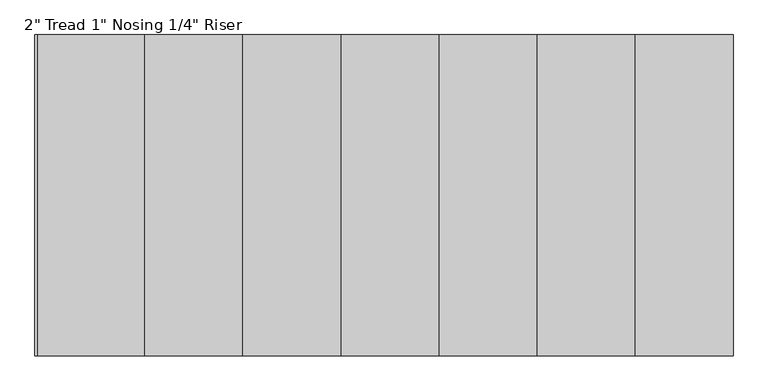
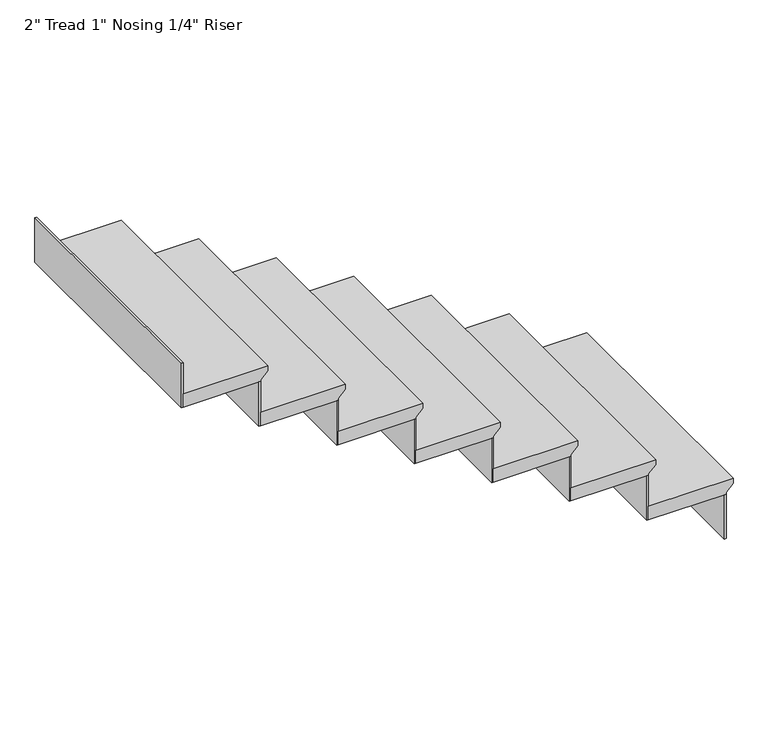
"""IFC4 building model written with IfcOpenShell, lengths in millimetres: stair flight geometry."""

from ifc_helpers import new_model, si_unit, frame, origin, place, context, project, spatial, polyline, outline, extrude, source, transform, mapped, element, save


def stair_flight_81020766(model_context):
    return source(origin(), model_context, "Body", "SweptSolid", [
        extrude(outline(polyline([(1862.6666667, -3900.6725091), (1862.6666667, -4205.4725091), (1811.8666667, -4205.4725091), (1811.8666667, -3926.0725091), (1818.2166667, -3926.0725091), (1843.6166667, -3900.6725091), (1862.6666667, -3900.6725091)])), frame((0.0, 8912.1149226, 0.0), z_axis=(0.0, 1.0, 0.0), x_axis=(0.0, 0.0, 1.0)), (0.0, 0.0, 1.0), 914.4),
        extrude(outline(polyline([(-3932.4225091, 9826.5149226), (-3926.0725091, 9826.5149226), (-3926.0725091, 8912.1149226), (-3932.4225091, 8912.1149226), (-3932.4225091, 9826.5149226)])), frame((0.0, 0.0, 1642.5333333), z_axis=(0.0, 0.0, 1.0), x_axis=(1.0, 0.0, 0.0)), (0.0, 0.0, 1.0), 169.3333333),
        extrude(outline(polyline([(-4211.8225091, 9826.5149226), (-4205.4725091, 9826.5149226), (-4205.4725091, 8912.1149226), (-4211.8225091, 8912.1149226), (-4211.8225091, 9826.5149226)])), frame((0.0, 0.0, 1811.8666667), z_axis=(0.0, 0.0, 1.0), x_axis=(1.0, 0.0, 0.0)), (0.0, 0.0, 1.0), 169.3333333),
        extrude(outline(polyline([(2032.0, -4180.0725091), (2032.0, -4484.8725091), (1981.2, -4484.8725091), (1981.2, -4205.4725091), (1987.55, -4205.4725091), (2012.95, -4180.0725091), (2032.0, -4180.0725091)])), frame((0.0, 8912.1149226, 0.0), z_axis=(0.0, 1.0, 0.0), x_axis=(0.0, 0.0, 1.0)), (0.0, 0.0, 1.0), 914.4),
        extrude(outline(polyline([(-4491.2225091, 9826.5149226), (-4484.8725091, 9826.5149226), (-4484.8725091, 8912.1149226), (-4491.2225091, 8912.1149226), (-4491.2225091, 9826.5149226)])), frame((0.0, 0.0, 1981.2), z_axis=(0.0, 0.0, 1.0), x_axis=(1.0, 0.0, 0.0)), (0.0, 0.0, 1.0), 169.3333333),
        extrude(outline(polyline([(2201.3333333, -4459.4725091), (2201.3333333, -4764.2725091), (2150.5333333, -4764.2725091), (2150.5333333, -4484.8725091), (2156.8833333, -4484.8725091), (2182.2833333, -4459.4725091), (2201.3333333, -4459.4725091)])), frame((0.0, 8912.1149226, 0.0), z_axis=(0.0, 1.0, 0.0), x_axis=(0.0, 0.0, 1.0)), (0.0, 0.0, 1.0), 914.4),
        extrude(outline(polyline([(-4770.6225091, 9826.5149226), (-4764.2725091, 9826.5149226), (-4764.2725091, 8912.1149226), (-4770.6225091, 8912.1149226), (-4770.6225091, 9826.5149226)])), frame((0.0, 0.0, 2150.5333333), z_axis=(0.0, 0.0, 1.0), x_axis=(1.0, 0.0, 0.0)), (0.0, 0.0, 1.0), 169.3333333),
        extrude(outline(polyline([(2370.6666667, -4738.8725091), (2370.6666667, -5043.6725091), (2319.8666667, -5043.6725091), (2319.8666667, -4764.2725091), (2326.2166667, -4764.2725091), (2351.6166667, -4738.8725091), (2370.6666667, -4738.8725091)])), frame((0.0, 8912.1149226, 0.0), z_axis=(0.0, 1.0, 0.0), x_axis=(0.0, 0.0, 1.0)), (0.0, 0.0, 1.0), 914.4),
        extrude(outline(polyline([(-5050.0225091, 9826.5149226), (-5043.6725091, 9826.5149226), (-5043.6725091, 8912.1149226), (-5050.0225091, 8912.1149226), (-5050.0225091, 9826.5149226)])), frame((0.0, 0.0, 2319.8666667), z_axis=(0.0, 0.0, 1.0), x_axis=(1.0, 0.0, 0.0)), (0.0, 0.0, 1.0), 169.3333333),
        extrude(outline(polyline([(2540.0, -5018.2725091), (2540.0, -5323.0725091), (2489.2, -5323.0725091), (2489.2, -5043.6725091), (2495.55, -5043.6725091), (2520.95, -5018.2725091), (2540.0, -5018.2725091)])), frame((0.0, 8912.1149226, 0.0), z_axis=(0.0, 1.0, 0.0), x_axis=(0.0, 0.0, 1.0)), (0.0, 0.0, 1.0), 914.4),
        extrude(outline(polyline([(-5329.4225091, 9826.5149226), (-5323.0725091, 9826.5149226), (-5323.0725091, 8912.1149226), (-5329.4225091, 8912.1149226), (-5329.4225091, 9826.5149226)])), frame((0.0, 0.0, 2489.2), z_axis=(0.0, 0.0, 1.0), x_axis=(1.0, 0.0, 0.0)), (0.0, 0.0, 1.0), 169.3333333),
        extrude(outline(polyline([(2709.3333333, -5297.6725091), (2709.3333333, -5602.4725091), (2658.5333333, -5602.4725091), (2658.5333333, -5323.0725091), (2664.8833333, -5323.0725091), (2690.2833333, -5297.6725091), (2709.3333333, -5297.6725091)])), frame((0.0, 8912.1149226, 0.0), z_axis=(0.0, 1.0, 0.0), x_axis=(0.0, 0.0, 1.0)), (0.0, 0.0, 1.0), 914.4),
        extrude(outline(polyline([(-5608.8225091, 9826.5149226), (-5602.4725091, 9826.5149226), (-5602.4725091, 8912.1149226), (-5608.8225091, 8912.1149226), (-5608.8225091, 9826.5149226)])), frame((0.0, 0.0, 2658.5333333), z_axis=(0.0, 0.0, 1.0), x_axis=(1.0, 0.0, 0.0)), (0.0, 0.0, 1.0), 169.3333333),
        extrude(outline(polyline([(2878.6666667, -5577.0725091), (2878.6666667, -5881.8725091), (2827.8666667, -5881.8725091), (2827.8666667, -5602.4725091), (2834.2166667, -5602.4725091), (2859.6166667, -5577.0725091), (2878.6666667, -5577.0725091)])), frame((0.0, 8912.1149226, 0.0), z_axis=(0.0, 1.0, 0.0), x_axis=(0.0, 0.0, 1.0)), (0.0, 0.0, 1.0), 914.4),
        extrude(outline(polyline([(-5888.2225091, 9826.5149226), (-5881.8725091, 9826.5149226), (-5881.8725091, 8912.1149226), (-5888.2225091, 8912.1149226), (-5888.2225091, 9826.5149226)])), frame((0.0, 0.0, 2827.8666667), z_axis=(0.0, 0.0, 1.0), x_axis=(1.0, 0.0, 0.0)), (0.0, 0.0, 1.0), 169.3333333),
    ])


if __name__ == "__main__":
    model = new_model("IFC4")
    model_context = context("Model", 3, world=origin())
    ifc_project = project(units=[si_unit("LENGTHUNIT", "METRE", prefix="MILLI")], contexts=[model_context])
    site = spatial("IfcSite", under=ifc_project)
    building = spatial("IfcBuilding", under=site)
    placement = place(None, origin())
    stair_flight_shape = stair_flight_81020766(model_context)
    element("IfcStairFlight", 1, ObjectType="2\" Tread 1\" Nosing 1/4\" Riser", at=placement, inside=building, context=model_context, shape_type="MappedRepresentation", body=[
        mapped(stair_flight_shape, transform((0.0, 0.0, 0.0), x_axis=(1.0, 0.0, 0.0), y_axis=(0.0, 1.0, 0.0), z_axis=(0.0, 0.0, 1.0))),
    ])
    save(model, "model.ifc")
